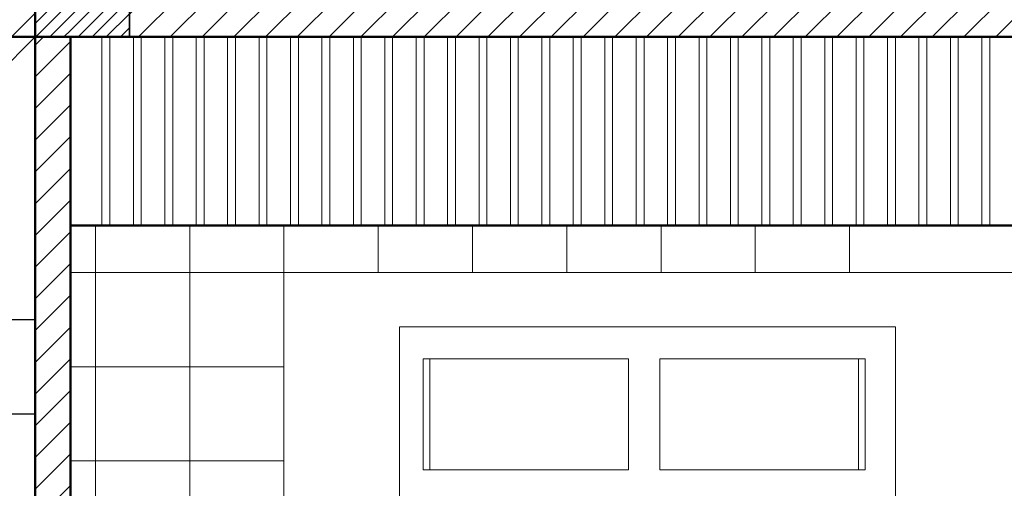
# Model space of a CAD drawing. Units: millimetres. Extents: x 225995 to 227247, y 225507 to 226008.
# Tile 8 of 23: x 226378 to 226504, y 225867 to 225927. Entities that reach past the tile are written whole.
import ezdxf

# ---------------------------------------------------------------- set-up
doc = ezdxf.new("R2010")
doc.units = ezdxf.units.MM
for name, color, linetype, lineweight in [('A-ANNO-DIMS', 2, 'Continuous', 18), ('A-COLS', 40, 'Continuous', 35), ('A-FLOR-PATT', 8, 'Continuous', 13), ('A-FLOR-STRS', 141, 'Continuous', 25), ('A-FURN', 9, 'Continuous', 18), ('A-WALL', 7, 'Continuous', 50), ('A-WALL-PATT', 8, 'Continuous', 13)]:
    doc.layers.add(name, color=color, linetype=linetype, lineweight=lineweight)
doc.styles.get("Standard").update_dxf_attribs({"font": 'arial.ttf'})
doc.dimstyles.new('ISO-25', dxfattribs={"dimtxt": 6, "dimasz": 2.5, "dimexe": 1.25, "dimexo": 0.625, "dimtad": 1, "dimdec": 0, "dimlunit": 3, "dimtxsty": 'Standard', "dimcen": 2.5, "dimadec": 0, "dimazin": 0, "dimtfac": 1, "dimtdec": 0, "dimtmove": 0, "dimatfit": 3, "dimfxl": 1, "dimarcsym": 0})
pattern_1 = [(45, (-6e-11, 234), (-0.898025612, 0.898025612), [])]

# ---------------------------------------------------------------- blocks, each defined once
blk = doc.blocks.new('A$C6D2A2628')
for p, q in [((0.291, 2.4297), (1.791, 2.4297)), ((0.291, 0.4297), (0.291, 2.4297)), ((1.791, 2.4297), (1.791, 0.4297)), ((0.3622, 2.3321), (0.9834, 2.3321)), ((0.3622, 1.9967), (0.3622, 2.3321)), ((0.3822, 1.9967), (0.3822, 2.3321)), ((0.9834, 2.3321), (0.9834, 1.9967)), ((1.0779, 2.3321), (1.6991, 2.3321)), ((1.0779, 1.9967), (1.0779, 2.3321)), ((1.6791, 2.3321), (1.6791, 1.9967)), ((1.6991, 2.3321), (1.6991, 1.9967)), ((0.9834, 1.9967), (0.3622, 1.9967)), ((1.6991, 1.9967), (1.0779, 1.9967))]:
    blk.add_line(p, q)
blk = doc.blocks.new('*D81')
at = {"layer": 'A-ANNO-DIMS', "color": 0, "lineweight": -2, "transparency": 16777216}
for p, q in [((226280.28, 225843.99), (226280.28, 225846.51)), ((226292.91, 225843.99), (226292.91, 225846.51)), ((226282.78, 225845.26), (226290.41, 225845.26)), ((226292.91, 225845.26), (226397.25, 225845.26))]:
    blk.add_line(p, q, dxfattribs=at)
at = {"layer": 'A-ANNO-DIMS', "color": 0, "transparency": 16777216}
for points in [[(226282.78, 225845.68), (226282.78, 225844.84), (226280.28, 225845.26)], [(226290.41, 225845.68), (226290.41, 225844.84), (226292.91, 225845.26)]]:
    blk.add_solid(points, dxfattribs=at)
at = {"layer": 'Defpoints', "color": 0, "transparency": 16777216}
for p in [(226292.91, 225845.26), (226280.28, 225843.36), (226292.91, 225843.36)]:
    blk.add_point(p, dxfattribs=at)
at = {"layer": 'A-ANNO-DIMS', "color": 0, "transparency": 16777216, "insert": (226346.33, 225848.99), "char_height": 6, "attachment_point": 5}
blk.add_mtext('BAR STOOL 1\'-0 1/2" TYP.', dxfattribs=at)

msp = doc.modelspace()

# ---------------------------------------------------------------- hatches: boundary and pattern name
at = {"layer": 'A-WALL-PATT'}
h = msp.add_hatch(dxfattribs=at)
h.set_pattern_fill('ANSI31', color=256, scale=0.9)
h.paths.add_polyline_path([(226380.38, 225933.77), (226374.38, 225933.77), (226374.38, 225924.77), (226380.38, 225924.77)])
h = msp.add_hatch(dxfattribs=at)
h.set_pattern_fill('ANSI31', color=256, scale=0.9)
h.paths.add_polyline_path([(226521.38, 225933.77), (226392.38, 225933.77), (226392.38, 225924.77), (226521.38, 225924.77)])
h = msp.add_hatch(dxfattribs=at)
h.set_pattern_fill('ANSI31', color=256, scale=0.4)
h.set_pattern_definition(pattern_1)
h.paths.add_polyline_path([(226384.88, 225929.27), (226380.38, 225929.27), (226380.38, 225924.77), (226384.88, 225924.77)])
h = msp.add_hatch(dxfattribs=at)
h.set_pattern_fill('ANSI31', color=256, scale=0.4)
h.set_pattern_definition(pattern_1)
h.paths.add_polyline_path([(226392.38, 225929.27), (226384.88, 225929.27), (226384.88, 225924.77), (226392.38, 225924.77)])
h = msp.add_hatch(dxfattribs=at)
h.set_pattern_fill('ANSI31', color=256, scale=0.9)
h.paths.add_polyline_path([(226384.88, 225924.77), (226380.38, 225924.77), (226380.38, 225817.91), (226384.88, 225817.91)])

# ---------------------------------------------------------------- linework, layer by layer
at = {"layer": 'A-COLS'}
msp.add_lwpolyline([(226380.38, 225924.77), (226380.38, 225933.77), (226392.38, 225933.77), (226392.38, 225924.77)], close=True, dxfattribs=at)
at = {"layer": 'A-FLOR-PATT'}
for p, q in [((226388.05, 225900.77), (226388.05, 225817.91)), ((226400.05, 225900.77), (226400.05, 225695.27)), ((226412.05, 225900.77), (226412.05, 225695.27)), ((226424.05, 225900.77), (226424.05, 225894.77)), ((226436.05, 225900.77), (226436.05, 225894.77)), ((226448.05, 225900.77), (226448.05, 225894.77)), ((226460.05, 225900.77), (226460.05, 225894.77)), ((226472.05, 225900.77), (226472.05, 225894.77)), ((226484.05, 225900.77), (226484.05, 225894.77)), ((226384.88, 225894.77), (226557.38, 225894.77)), ((226384.88, 225882.77), (226412.05, 225882.77)), ((226384.88, 225870.77), (226412.05, 225870.77))]:
    msp.add_line(p, q, dxfattribs=at)
at = {"layer": 'A-FLOR-STRS'}
for p, q in [((226344.38, 225888.77), (226380.38, 225924.77)), ((226248.38, 225888.77), (226380.38, 225888.77)), ((226344.38, 225876.77), (226380.38, 225876.77))]:
    msp.add_line(p, q, dxfattribs=at)
at = {"layer": 'A-FURN'}
for p, q in [((226388.88, 225900.77), (226388.88, 225924.77)), ((226389.88, 225900.77), (226389.88, 225924.77)), ((226392.88, 225900.77), (226392.88, 225924.77)), ((226393.88, 225900.77), (226393.88, 225924.77)), ((226396.88, 225900.77), (226396.88, 225924.77)), ((226397.88, 225900.77), (226397.88, 225924.77)), ((226400.88, 225900.77), (226400.88, 225924.77)), ((226401.88, 225900.77), (226401.88, 225924.77)), ((226404.88, 225900.77), (226404.88, 225924.77)), ((226405.88, 225900.77), (226405.88, 225924.77)), ((226408.88, 225900.77), (226408.88, 225924.77)), ((226409.88, 225900.77), (226409.88, 225924.77)), ((226412.88, 225900.77), (226412.88, 225924.77)), ((226413.88, 225900.77), (226413.88, 225924.77)), ((226416.88, 225900.77), (226416.88, 225924.77)), ((226417.88, 225900.77), (226417.88, 225924.77)), ((226420.88, 225900.77), (226420.88, 225924.77)), ((226421.88, 225900.77), (226421.88, 225924.77)), ((226424.88, 225900.77), (226424.88, 225924.77)), ((226425.88, 225900.77), (226425.88, 225924.77)), ((226428.88, 225900.77), (226428.88, 225924.77)), ((226429.88, 225900.77), (226429.88, 225924.77)), ((226432.88, 225900.77), (226432.88, 225924.77)), ((226433.88, 225900.77), (226433.88, 225924.77)), ((226436.88, 225900.77), (226436.88, 225924.77)), ((226437.88, 225900.77), (226437.88, 225924.77)), ((226440.88, 225900.77), (226440.88, 225924.77)), ((226441.88, 225900.77), (226441.88, 225924.77)), ((226444.88, 225900.77), (226444.88, 225924.77)), ((226445.88, 225900.77), (226445.88, 225924.77)), ((226448.88, 225900.77), (226448.88, 225924.77)), ((226449.88, 225900.77), (226449.88, 225924.77)), ((226452.88, 225900.77), (226452.88, 225924.77)), ((226453.88, 225900.77), (226453.88, 225924.77)), ((226456.88, 225900.77), (226456.88, 225924.77)), ((226457.88, 225900.77), (226457.88, 225924.77)), ((226460.88, 225900.77), (226460.88, 225924.77)), ((226461.88, 225900.77), (226461.88, 225924.77)), ((226464.88, 225900.77), (226464.88, 225924.77)), ((226465.88, 225900.77), (226465.88, 225924.77)), ((226468.88, 225900.77), (226468.88, 225924.77)), ((226469.88, 225900.77), (226469.88, 225924.77)), ((226472.88, 225900.77), (226472.88, 225924.77)), ((226473.88, 225900.77), (226473.88, 225924.77)), ((226476.88, 225900.77), (226476.88, 225924.77)), ((226477.88, 225900.77), (226477.88, 225924.77)), ((226480.88, 225900.77), (226480.88, 225924.77)), ((226481.88, 225900.77), (226481.88, 225924.77)), ((226484.88, 225900.77), (226484.88, 225924.77)), ((226485.88, 225900.77), (226485.88, 225924.77)), ((226488.88, 225900.77), (226488.88, 225924.77)), ((226489.88, 225900.77), (226489.88, 225924.77)), ((226492.88, 225900.77), (226492.88, 225924.77)), ((226493.88, 225900.77), (226493.88, 225924.77)), ((226496.88, 225900.77), (226496.88, 225924.77)), ((226497.88, 225900.77), (226497.88, 225924.77)), ((226500.88, 225900.77), (226500.88, 225924.77)), ((226501.88, 225900.77), (226501.88, 225924.77))]:
    msp.add_line(p, q, dxfattribs=at)
at = {"layer": 'A-WALL'}
for p, q in [((226380.38, 225933.77), (226380.38, 225924.77)), ((226236.38, 225924.77), (226557.38, 225924.77)), ((226248.38, 225924.77), (226380.38, 225924.77)), ((226380.38, 225740.27), (226380.38, 225924.77)), ((226380.38, 225924.77), (226380.38, 225740.27)), ((226384.88, 225740.27), (226384.88, 225924.77)), ((226384.88, 225924.77), (226557.38, 225924.77)), ((226384.88, 225740.27), (226384.88, 225924.77)), ((226384.88, 225900.77), (226557.38, 225900.77))]:
    msp.add_line(p, q, dxfattribs=at)

# ---------------------------------------------------------------- block references
at = {"layer": 'A-FURN', "xscale": 42.09102840542158, "yscale": 42.09102840542158, "zscale": 42.09102840542158}
msp.add_blockref('A$C6D2A2628', (226414.51, 225785.59), dxfattribs=at)

# ---------------------------------------------------------------- dimensions: what is measured, and where the dimension line sits
at = {"layer": 'A-ANNO-DIMS'}
dim = msp.add_linear_dim(base=(226292.91, 225845.26), p1=(226280.28, 225843.36), p2=(226292.91, 225843.36), text='BAR STOOL <> TYP.', dimstyle='ISO-25', override={"dimdec": 1, "dimrnd": 0, "dimzin": 1, "dimlunit": 4, "dimfrac": 2}, dxfattribs=at)
dim.commit()
dim.dimension.update_dxf_attribs({"geometry": '*D81', "text_midpoint": (226346.33, 225848.99)})

doc.saveas('drawing.dxf')
